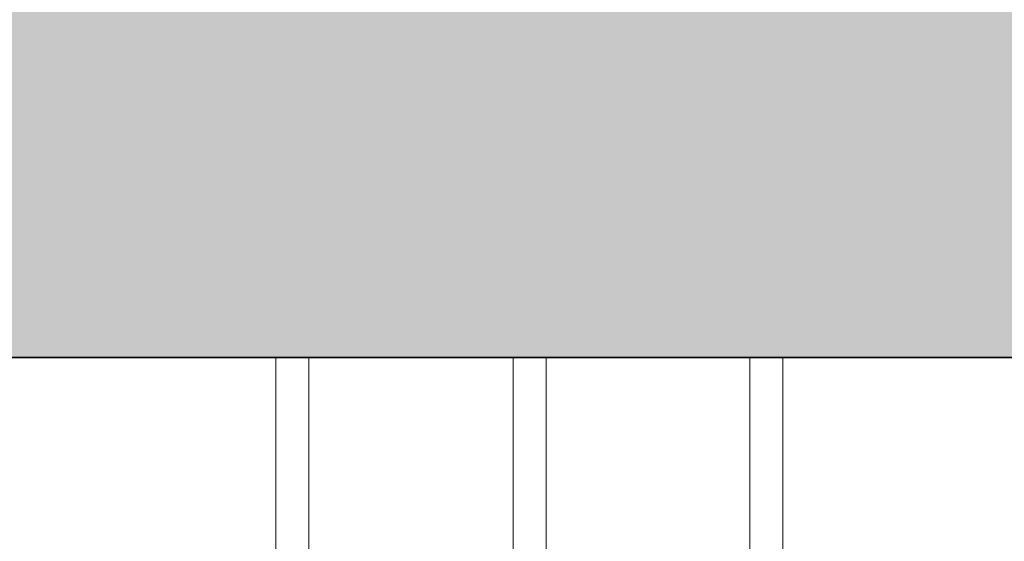
# Model space of a CAD drawing. Units: inches. Extents: x 2696 to 3240, y 1564 to 2310.
# Tile 20 of 76: x 2783.067 to 2792.41, y 1904.955 to 1909.906. Entities that reach past the tile are written whole.
import ezdxf

# ---------------------------------------------------------------- set-up
doc = ezdxf.new("R2010")
doc.units = ezdxf.units.IN
for name, color, linetype, lineweight in [('A-ANNO-DIMS', 3, 'Continuous', 18), ('A-FLOR-FIXT', 8, 'Continuous', 18), ('A-FURN', 251, 'Continuous', 13), ('A-WALL', 7, 'Continuous', 35), ('A-WALL-PATT', 9, 'Continuous', 13)]:
    doc.layers.add(name, color=color, linetype=linetype, lineweight=lineweight)
doc.layers.add('FURNITURE', color=250, linetype='Continuous')
doc.styles.add('TIMES NEW', font='times.ttf')
doc.dimstyles.new('Siddhuu', dxfattribs={"dimtxt": 6, "dimasz": 2.5, "dimexe": 1.25, "dimexo": 0.625, "dimtad": 1, "dimdec": 1, "dimlunit": 4, "dimtxsty": 'TIMES NEW', "dimcen": 2.5, "dimclrd": 256, "dimclre": 1, "dimclrt": 7, "dimadec": 0, "dimazin": 0, "dimtfac": 1, "dimtdec": 1, "dimtmove": 0, "dimatfit": 3, "dimfxl": 1, "dimtolj": 1, "dimlwd": -1, "dimarcsym": 0})

# ---------------------------------------------------------------- blocks, each defined once
blk = doc.blocks.new('A$C1af1f523')
at = {"layer": 'A-FURN'}
for p, q in [((0, 2.5605), (-4.2116, 2.5605)), ((0, 2.5605, 0.5), (-4.2116, 2.5605, 0.5)), ((0, 2.248), (-4.2116, 2.248)), ((0, 2.248, 0.5), (-4.2116, 2.248, 0.5)), ((0, 0.3125), (-6.5015, 0.3125)), ((0, 0.3125, 0.5), (-6.5015, 0.3125, 0.5)), ((0, 0), (-6.5015, 0)), ((0, 0, 0.5), (-6.5015, 0, 0.5)), ((0, -1.9388), (-4.2094, -1.9388)), ((0, -1.9388, 0.5), (-4.2094, -1.9388, 0.5)), ((0, -2.2513), (-4.2094, -2.2513)), ((0, -2.2513, 0.5), (-4.2094, -2.2513, 0.5))]:
    blk.add_line(p, q, dxfattribs=at)
at = {"layer": 'FURNITURE'}
for p, q in [((0, 2.5605), (0, 2.5605, 0.5)), ((0, 2.248), (0, 2.248, 0.5)), ((0, 0.3125), (0, 0.3125, 0.5)), ((0, 0), (0, 0, 0.5)), ((0, -1.9388), (0, -1.9388, 0.5)), ((0, -2.2513), (0, -2.2513, 0.5))]:
    blk.add_line(p, q, dxfattribs=at)
at = {"layer": 'A-FURN'}
mesh = blk.add_polyface(dxfattribs=at)
corners = [(0, 2.5605, 0.5), (-4.2116, 2.5605), (-4.2116, 2.5605, 0.5), (0, 2.5605)]
mesh.append_faces([[corners[k] for k in face] for face in [(2, 1, 0), (3, 0, 1)]], dxfattribs={"vtx1": -1})
mesh = blk.add_polyface(dxfattribs=at)
corners = [(0, 2.248, 0.5), (-4.2116, 2.248), (-4.2116, 2.248, 0.5), (0, 2.248)]
mesh.append_faces([[corners[k] for k in face] for face in [(2, 1, 0), (3, 0, 1)]], dxfattribs={"vtx1": -1})
mesh = blk.add_polyface(dxfattribs=at)
corners = [(0, 0.3125, 0.5), (-6.5015, 0.3125), (-6.5015, 0.3125, 0.5), (0, 0.3125)]
mesh.append_faces([[corners[k] for k in face] for face in [(2, 1, 0), (3, 0, 1)]], dxfattribs={"vtx1": -1})
mesh = blk.add_polyface(dxfattribs=at)
corners = [(0, 0, 0.5), (-6.5015, 0), (-6.5015, 0, 0.5), (0, 0)]
mesh.append_faces([[corners[k] for k in face] for face in [(2, 1, 0), (3, 0, 1)]], dxfattribs={"vtx1": -1})
mesh = blk.add_polyface(dxfattribs=at)
corners = [(0, -1.9388, 0.5), (-4.2094, -1.9388), (-4.2094, -1.9388, 0.5), (0, -1.9388)]
mesh.append_faces([[corners[k] for k in face] for face in [(2, 1, 0), (3, 0, 1)]], dxfattribs={"vtx1": -1})
mesh = blk.add_polyface(dxfattribs=at)
corners = [(0, -2.2513, 0.5), (-4.2094, -2.2513), (-4.2094, -2.2513, 0.5), (0, -2.2513)]
mesh.append_faces([[corners[k] for k in face] for face in [(2, 1, 0), (3, 0, 1)]], dxfattribs={"vtx1": -1})
blk = doc.blocks.new('*D55')
at = {"layer": 'A-ANNO-DIMS', "color": 1, "lineweight": -2, "transparency": 16777216}
for p, q in [((3189.9864, 1980.2011), (2709.3614, 1980.2011)), ((3189.9864, 1893.2011), (2709.3614, 1893.2011))]:
    blk.add_line(p, q, dxfattribs=at)
at = {"layer": 'A-ANNO-DIMS', "transparency": 16777216}
blk.add_line((2710.6114, 1895.7011), (2710.6114, 1977.7011), dxfattribs=at)
for points in [[(2710.1947, 1977.7011), (2711.0281, 1977.7011), (2710.6114, 1980.2011)], [(2710.1947, 1895.7011), (2711.0281, 1895.7011), (2710.6114, 1893.2011)]]:
    blk.add_solid(points, dxfattribs=at)
at = {"layer": 'Defpoints', "color": 0, "transparency": 16777216}
for p in [(2710.6114, 1980.2011), (3190.6114, 1980.2011), (3190.6114, 1893.2011)]:
    blk.add_point(p, dxfattribs=at)
at = {"layer": 'A-ANNO-DIMS', "color": 7, "transparency": 16777216, "insert": (2706.9258, 1936.7011), "char_height": 6, "attachment_point": 5, "rotation": 90, "style": 'TIMES NEW'}
blk.add_mtext('\\A1;7\'-3"', dxfattribs=at)
blk = doc.blocks.new('*D57')
at = {"layer": 'A-ANNO-DIMS', "color": 1, "lineweight": -2, "transparency": 16777216}
for p, q in [((2754.6114, 2018.5761), (2754.6114, 1568.9511)), ((2956.7088, 2018.5761), (2956.7088, 1568.9511))]:
    blk.add_line(p, q, dxfattribs=at)
at = {"layer": 'A-ANNO-DIMS', "transparency": 16777216}
blk.add_line((2757.1114, 1570.2011), (2954.2088, 1570.2011), dxfattribs=at)
for points in [[(2757.1114, 1570.6178), (2757.1114, 1569.7844), (2754.6114, 1570.2011)], [(2954.2088, 1570.6178), (2954.2088, 1569.7844), (2956.7088, 1570.2011)]]:
    blk.add_solid(points, dxfattribs=at)
at = {"layer": 'Defpoints', "color": 0, "transparency": 16777216}
for p in [(2754.6114, 2019.2011), (2956.7088, 2019.2011), (2956.7088, 1570.2011)]:
    blk.add_point(p, dxfattribs=at)
at = {"layer": 'A-ANNO-DIMS', "color": 7, "transparency": 16777216, "insert": (2855.6601, 1573.878), "char_height": 6, "attachment_point": 5, "style": 'TIMES NEW'}
blk.add_mtext('\\A1;16\'-10"', dxfattribs=at)
blk = doc.blocks.new('*D78')
at = {"layer": 'A-ANNO-DIMS', "transparency": 16777216}
for p, q in [((2710.6114, 1901.7011), (2710.6114, 1935.1007)), ((2710.6114, 1895.7011), (2710.6114, 1899.2011))]:
    blk.add_line(p, q, dxfattribs=at)
at = {"layer": 'A-ANNO-DIMS', "color": 1, "lineweight": -2, "transparency": 16777216}
for p, q in [((3189.9864, 1901.7011), (2709.3614, 1901.7011)), ((3189.9864, 1893.2011), (2709.3614, 1893.2011))]:
    blk.add_line(p, q, dxfattribs=at)
at = {"layer": 'A-ANNO-DIMS', "transparency": 16777216}
for points in [[(2710.1947, 1899.2011), (2711.0281, 1899.2011), (2710.6114, 1901.7011)], [(2710.1947, 1895.7011), (2711.0281, 1895.7011), (2710.6114, 1893.2011)]]:
    blk.add_solid(points, dxfattribs=at)
at = {"layer": 'Defpoints', "color": 0, "transparency": 16777216}
for p in [(2710.6114, 1901.7011), (3190.6114, 1901.7011), (3190.6114, 1893.2011)]:
    blk.add_point(p, dxfattribs=at)
at = {"layer": 'A-ANNO-DIMS', "color": 7, "transparency": 16777216, "insert": (2706.8501, 1919.6509), "char_height": 6, "attachment_point": 5, "rotation": 90, "style": 'TIMES NEW'}
blk.add_mtext('\\A1;0\'-8 1/2"', dxfattribs=at)

msp = doc.modelspace()

# ---------------------------------------------------------------- hatches: boundary and pattern name
at = {"layer": 'A-WALL-PATT', "transparency": 33554556}
h = msp.add_hatch(color=256, dxfattribs=at)
h.dxf.hatch_style = 1
h.paths.add_polyline_path([(2879.1114, 2253.2011), (2905.9101, 2253.2011), (2905.9101, 2262.2011), (2841.889, 2262.2011), (2841.889, 2253.2011), (2870.1114, 2253.2011), (2870.1114, 2176.6011), (2965.7088, 2176.6011), (2965.7088, 2206.7011), (2973.5828, 2206.7011), (2973.5828, 2215.7011), (2965.7088, 2215.7011), (2965.7088, 2262.2011), (2929.9101, 2262.2011), (2929.9101, 2253.2011), (2956.7088, 2253.2011), (2956.7088, 2185.6011), (2879.1114, 2185.6011)])
h.paths.add_polyline_path([(2782.8338, 2262.2011), (2745.6114, 2262.2011), (2745.6114, 2228.7287), (2754.6114, 2228.7287), (2754.6114, 2253.2011), (2782.8338, 2253.2011)])
h.paths.add_polyline_path([(2754.6114, 2136.2011), (2965.7088, 2136.2011), (2965.7088, 2145.2011), (2879.1114, 2145.2011), (2879.1114, 2147.0735), (2877.3397, 2147.0735), (2870.1114, 2147.0735), (2870.1114, 2145.2011), (2754.6114, 2145.2011), (2754.6114, 2169.6735), (2745.6114, 2169.6735), (2745.6114, 2000.2011), (2754.6114, 2000.2011), (2754.6114, 2019.2011), (2849.0828, 2019.2011), (2849.0828, 2023.7011), (2841.2088, 2023.7011), (2841.2088, 2051.8271), (2836.7088, 2051.8271), (2836.7088, 2023.7011), (2754.6114, 2023.7011), (2754.6114, 2091.2011), (2836.7088, 2091.2011), (2836.7088, 2087.8271), (2841.2088, 2087.8271), (2841.2088, 2095.7011), (2754.6114, 2095.7011)])
h.paths.add_polyline_path([(2965.7088, 2136.2011), (2956.7088, 2136.2011), (2956.7088, 2023.7011), (2885.0828, 2023.7011), (2885.0828, 2019.2011), (2956.7088, 2019.2011), (2956.7088, 1950.5751), (2965.7088, 1950.5751), (2965.7088, 1980.2011), (2973.5828, 1980.2011), (2973.5828, 1989.2011), (2965.7088, 1989.2011)])
h.paths.add_polyline_path([(2754.6114, 1906.7011), (2880.2088, 1906.7011), (2884.7088, 1906.7011), (2956.7088, 1906.7011), (2956.7088, 1792.7011), (2944.7088, 1792.7011), (2944.7088, 1783.7011), (2956.7088, 1783.7011), (2956.7088, 1740.2011), (2884.7088, 1740.2011), (2884.7088, 1783.7011), (2896.7088, 1783.7011), (2896.7088, 1792.7011), (2884.7088, 1792.7011), (2884.7088, 1846.7011), (2880.2088, 1846.7011), (2880.2088, 1740.2011), (2754.6114, 1740.2011), (2754.6114, 1777.2011), (2745.6114, 1777.2011), (2745.6114, 1692.7011), (2754.6114, 1692.7011), (2754.6114, 1731.2011), (2956.7088, 1731.2011), (2956.7088, 1723.3271), (2965.7088, 1723.3271), (2965.7088, 1884.2011), (2973.5828, 1884.2011), (2973.5828, 1893.2011), (2965.7088, 1893.2011), (2965.7088, 1914.5751), (2956.7088, 1914.5751), (2956.7088, 1911.2011), (2754.6114, 1911.2011), (2754.6114, 1930.2011), (2745.6114, 1930.2011), (2745.6114, 1817.2011), (2754.6114, 1817.2011), (2754.6114, 1854.2011), (2826.6114, 1854.2011), (2826.6114, 1868.8271), (2822.1114, 1868.8271), (2822.1114, 1858.7011), (2754.6114, 1858.7011)])
h.paths.add_polyline_path([(2965.7088, 1656.2011), (3008.2374, 1656.2011), (3008.2374, 1665.2011), (2965.7088, 1665.2011), (2965.7088, 1693.3271), (2956.7088, 1693.3271), (2956.7088, 1686.2011), (2934.5828, 1686.2011), (2934.5828, 1681.7011), (2956.7088, 1681.7011), (2956.7088, 1614.2011), (2896.7088, 1614.2011), (2896.7088, 1681.7011), (2904.5828, 1681.7011), (2904.5828, 1686.2011), (2892.2088, 1686.2011), (2892.2088, 1614.2011), (2858.4101, 1614.2011), (2858.4101, 1605.2011), (2965.7088, 1605.2011)])
h.paths.add_polyline_path([(2788.4101, 1614.2011), (2754.6114, 1614.2011), (2754.6114, 1652.7011), (2745.6114, 1652.7011), (2745.6114, 1605.2011), (2788.4101, 1605.2011)])
h.paths.add_polyline_path([(3199.6114, 1633.0476), (3190.6114, 1633.0476), (3190.6114, 1614.2011), (3082.6114, 1614.2011), (3082.6114, 1665.2011), (3070.2374, 1665.2011), (3070.2374, 1656.2011), (3078.1114, 1656.2011), (3078.1114, 1605.2011), (3199.6114, 1605.2011)])
h.paths.add_polyline_path([(3199.6114, 1702.0476), (3190.6114, 1702.0476), (3190.6114, 1699.7011), (3106.6114, 1699.7011), (3106.6114, 1747.7011), (3190.6114, 1747.7011), (3190.6114, 1752.2011), (3082.6114, 1752.2011), (3082.6114, 1760.0751), (3078.1114, 1760.0751), (3078.1114, 1747.7011), (3102.1114, 1747.7011), (3102.1114, 1699.7011), (3078.1114, 1699.7011), (3078.1114, 1695.2011), (3190.6114, 1695.2011), (3190.6114, 1676.3546), (3199.6114, 1676.3546)])
h.paths.add_polyline_path([(3199.6114, 1783.2011), (3190.6114, 1783.2011), (3190.6114, 1745.3546), (3199.6114, 1745.3546)])
h.paths.add_polyline_path([(3082.6114, 1884.2011), (3190.6114, 1884.2011), (3190.6114, 1853.2011), (3199.6114, 1853.2011), (3199.6114, 1901.7011), (3190.6114, 1901.7011), (3190.6114, 1893.2011), (3005.5828, 1893.2011), (3005.5828, 1891.2811), (3005.5828, 1884.2011), (3078.1114, 1884.2011), (3078.1114, 1792.0751), (3082.6114, 1792.0751)])
h.paths.add_polyline_path([(3199.6114, 1994.7011), (3190.6114, 1994.7011), (3190.6114, 1989.2011), (3073.7088, 1989.2011), (3073.7088, 2034.2011), (3069.2088, 2034.2011), (3069.2088, 1989.2011), (3005.5828, 1989.2011), (3005.5828, 1980.2011), (3190.6114, 1980.2011), (3190.6114, 1971.7011), (3199.6114, 1971.7011)])
h.paths.add_polyline_path([(3199.6114, 2155.2011), (3190.6114, 2155.2011), (3190.6114, 2064.7011), (3199.6114, 2064.7011)])
h.paths.add_polyline_path([(3190.6114, 2074.7011), (3106.6114, 2074.7011), (3106.6114, 2122.7011), (3190.6114, 2122.7011), (3190.6114, 2127.2011), (3082.7088, 2127.2011), (3082.7088, 2135.0751), (3073.7088, 2135.0751), (3073.7088, 2122.7011), (3102.1114, 2122.7011), (3102.1114, 2074.7011), (3069.2088, 2074.7011), (3069.2088, 2070.2011), (3190.6114, 2070.2011)])
h.paths.add_polyline_path([(3082.7088, 2253.2011), (3190.6114, 2253.2011), (3190.6114, 2225.2011), (3199.6114, 2225.2011), (3199.6114, 2262.2011), (3073.7088, 2262.2011), (3073.7088, 2215.7011), (3035.5828, 2215.7011), (3035.5828, 2206.7011), (3073.7088, 2206.7011), (3073.7088, 2171.0751), (3082.7088, 2171.0751)])

# ---------------------------------------------------------------- linework, layer by layer
at = {"layer": 'A-WALL'}
msp.add_line((2754.6114, 1906.7011), (2880.2088, 1906.7011), dxfattribs=at)

# ---------------------------------------------------------------- block references
at = {"layer": 'A-FLOR-FIXT', "xscale": -1, "rotation": 270}
msp.add_blockref('A$C1af1f523', (2787.7487, 1906.7011), dxfattribs=at)

# ---------------------------------------------------------------- dimensions: what is measured, and where the dimension line sits
at = {"layer": 'A-ANNO-DIMS'}
dim = msp.add_linear_dim(base=(2956.7088, 1570.2011), p1=(2754.6114, 2019.2011), p2=(2956.7088, 2019.2011), dimstyle='Siddhuu', override={"dimdec": 1, "dimlfac": 1, "dimrnd": 0, "dimzin": 1, "dimdsep": 46, "dimlunit": 4, "dimfrac": 2}, dxfattribs=at)
dim.commit()
dim.dimension.update_dxf_attribs({"geometry": '*D57', "text_midpoint": (2855.6601, 1573.878)})
for base, p2, picture, middle in [((2710.6114, 1980.2011), (3190.6114, 1980.2011), '*D55', (2706.9258, 1936.7011)), ((2710.6114, 1901.7011), (3190.6114, 1901.7011), '*D78', (2706.8501, 1919.6509))]:
    dim = msp.add_linear_dim(base=base, p1=(3190.6114, 1893.2011), p2=p2, angle=90, dimstyle='Siddhuu', override={"dimdec": 1, "dimlfac": 1, "dimrnd": 0, "dimzin": 1, "dimdsep": 46, "dimlunit": 4, "dimfrac": 2}, dxfattribs=at)
    dim.commit()
    dim.dimension.update_dxf_attribs({"geometry": picture, "text_midpoint": middle})

doc.saveas('drawing.dxf')
